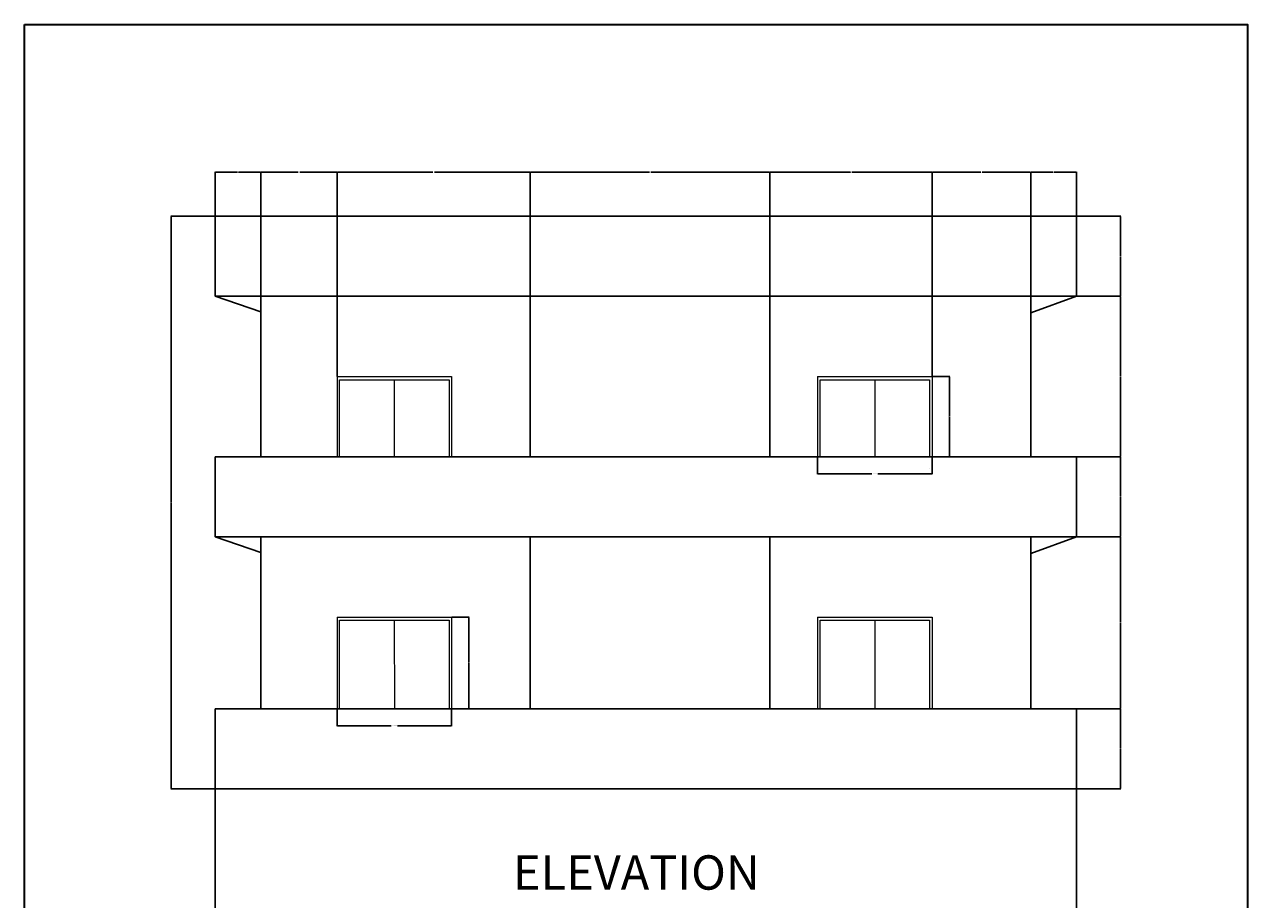
# Model space of a CAD drawing. Units: inches. Extents: x 1854 to 2495, y 1460 to 2772.
# Tile 12 of 12: x 1854 to 2495, y 2314 to 2772. Entities that reach past the tile are written whole.
import ezdxf

# ---------------------------------------------------------------- set-up
doc = ezdxf.new("R2010")
doc.units = ezdxf.units.IN
for name, color, linetype, lineweight in [('A-ANNO-DIMS', 2, 'Continuous', 18), ('A-ANNO-TEXT', 7, 'Continuous', 25), ('A-ANNO-TTLB', 7, 'Continuous', 35), ('A-ELEV', 7, 'Continuous', 25), ('A-ELEV-GLAZ', 4, 'Continuous', 18)]:
    doc.layers.add(name, color=color, linetype=linetype, lineweight=lineweight)
doc.styles.get("Standard").update_dxf_attribs({"font": 'arial.ttf'})
doc.dimstyles.get("Standard").update_dxf_attribs({"dimtxt": 0.18, "dimasz": 0.18, "dimexe": 0.18, "dimexo": 0.0625, "dimgap": 0.09, "dimtad": 0, "dimtih": 1, "dimtoh": 1, "dimdec": 4, "dimzin": 0, "dimdsep": 46, "dimtxsty": 'Standard', "dimcen": 0.09, "dimadec": 0, "dimazin": 0, "dimtfac": 1, "dimtdec": 4, "dimtofl": 0, "dimtmove": 0, "dimatfit": 3, "dimfxl": 1, "dimtolj": 1, "dimtzin": 0, "dimarcsym": 0})

# ---------------------------------------------------------------- blocks, each defined once
blk = doc.blocks.new('ELEV-WINDOW-60X48')
for p, q in [((0, 48), (0, 0)), ((0, 48), (60, 48)), ((29.95, 46.33), (30, 0)), ((60, 48), (60, 0)), ((0, 0), (60, 0))]:
    blk.add_line(p, q)
blk.add_lwpolyline([(1.27, 46.33), (58.63, 46.33), (58.63, 0), (1.27, 0)], close=True)
blk = doc.blocks.new('ELEV-WINDOW-60X42')
for p, q in [((0, 42), (0, 0)), ((0, 42), (60, 42)), ((29.95, 40.33), (29.99, 0)), ((60, 42), (60, 0))]:
    blk.add_line(p, q)
blk.add_lwpolyline([(1.27, 0), (1.27, 40.33), (58.63, 40.33), (58.63, 0)])
blk = doc.blocks.new('*D27')
at = {"layer": 'A-ANNO-DIMS', "color": 0, "lineweight": -2, "transparency": 16777216}
for p, q in [((2017.83, 2414.03), (2017.83, 2404.91)), ((2077.83, 2414.03), (2077.83, 2404.91)), ((2018.01, 2405.09), (2046.22, 2405.09)), ((2077.65, 2405.09), (2049.44, 2405.09))]:
    blk.add_line(p, q, dxfattribs=at)
at = {"layer": 'A-ANNO-DIMS', "color": 0, "transparency": 16777216}
for points in [[(2018.01, 2405.12), (2018.01, 2405.06), (2017.83, 2405.09)], [(2077.65, 2405.12), (2077.65, 2405.06), (2077.83, 2405.09)]]:
    blk.add_solid(points, dxfattribs=at)
at = {"layer": 'Defpoints', "color": 0, "transparency": 16777216}
for p in [(2017.83, 2414.09), (2077.83, 2414.09), (2077.83, 2405.09)]:
    blk.add_point(p, dxfattribs=at)
at = {"layer": 'A-ANNO-DIMS', "color": 0, "transparency": 16777216, "insert": (2047.83, 2405.09), "char_height": 0.18, "attachment_point": 5}
blk.add_mtext('\\A1;LOWER WINDOW 60 TYP.', dxfattribs=at)
blk = doc.blocks.new('*D28')
at = {"layer": 'A-ANNO-DIMS', "color": 0, "lineweight": -2, "transparency": 16777216}
for p, q in [((2077.89, 2462.09), (2087.01, 2462.09)), ((2086.83, 2461.91), (2086.83, 2438.27)), ((2086.83, 2414.27), (2086.83, 2437.91)), ((2077.89, 2414.09), (2087.01, 2414.09))]:
    blk.add_line(p, q, dxfattribs=at)
at = {"layer": 'A-ANNO-DIMS', "color": 0, "transparency": 16777216}
for points in [[(2086.8, 2461.91), (2086.86, 2461.91), (2086.83, 2462.09)], [(2086.8, 2414.27), (2086.86, 2414.27), (2086.83, 2414.09)]]:
    blk.add_solid(points, dxfattribs=at)
at = {"layer": 'Defpoints', "color": 0, "transparency": 16777216}
for p in [(2077.83, 2462.09), (2086.83, 2462.09), (2077.83, 2414.09)]:
    blk.add_point(p, dxfattribs=at)
at = {"layer": 'A-ANNO-DIMS', "color": 0, "transparency": 16777216, "insert": (2086.83, 2438.09), "char_height": 0.18, "attachment_point": 5}
blk.add_mtext('\\A1;48 TYP.', dxfattribs=at)
blk = doc.blocks.new('*D29')
at = {"layer": 'A-ANNO-DIMS', "color": 0, "lineweight": -2, "transparency": 16777216}
for p, q in [((2269.45, 2546.03), (2269.45, 2536.91)), ((2329.45, 2546.03), (2329.45, 2536.91)), ((2269.63, 2537.09), (2297.87, 2537.09)), ((2329.27, 2537.09), (2301.02, 2537.09))]:
    blk.add_line(p, q, dxfattribs=at)
at = {"layer": 'A-ANNO-DIMS', "color": 0, "transparency": 16777216}
for points in [[(2269.63, 2537.12), (2269.63, 2537.06), (2269.45, 2537.09)], [(2329.27, 2537.12), (2329.27, 2537.06), (2329.45, 2537.09)]]:
    blk.add_solid(points, dxfattribs=at)
at = {"layer": 'Defpoints', "color": 0, "transparency": 16777216}
for p in [(2269.45, 2546.09), (2329.45, 2546.09), (2329.45, 2537.09)]:
    blk.add_point(p, dxfattribs=at)
at = {"layer": 'A-ANNO-DIMS', "color": 0, "transparency": 16777216, "insert": (2299.45, 2537.09), "char_height": 0.18, "attachment_point": 5}
blk.add_mtext('\\A1;UPPER WINDOW 60 TYP.', dxfattribs=at)
blk = doc.blocks.new('*D30')
at = {"layer": 'A-ANNO-DIMS', "color": 0, "lineweight": -2, "transparency": 16777216}
for p, q in [((2329.51, 2588.09), (2338.63, 2588.09)), ((2338.45, 2587.91), (2338.45, 2567.27)), ((2338.45, 2546.27), (2338.45, 2566.91)), ((2329.51, 2546.09), (2338.63, 2546.09))]:
    blk.add_line(p, q, dxfattribs=at)
at = {"layer": 'A-ANNO-DIMS', "color": 0, "transparency": 16777216}
for points in [[(2338.42, 2587.91), (2338.48, 2587.91), (2338.45, 2588.09)], [(2338.42, 2546.27), (2338.48, 2546.27), (2338.45, 2546.09)]]:
    blk.add_solid(points, dxfattribs=at)
at = {"layer": 'Defpoints', "color": 0, "transparency": 16777216}
for p in [(2329.45, 2588.09), (2338.45, 2588.09), (2329.45, 2546.09)]:
    blk.add_point(p, dxfattribs=at)
at = {"layer": 'A-ANNO-DIMS', "color": 0, "transparency": 16777216, "insert": (2338.45, 2567.09), "char_height": 0.18, "attachment_point": 5}
blk.add_mtext('\\A1;42 TYP.', dxfattribs=at)
blk = doc.blocks.new('*D74')
at = {"layer": 'A-ANNO-DIMS', "color": 0, "lineweight": -2, "transparency": 16777216}
for p, q in [((1953.98, 2372.03), (1953.98, 2284.46)), ((2404.98, 2372.03), (2404.98, 2284.46)), ((1954.16, 2284.64), (2179.21, 2284.64)), ((2404.8, 2284.64), (2179.76, 2284.64))]:
    blk.add_line(p, q, dxfattribs=at)
at = {"layer": 'A-ANNO-DIMS', "color": 0, "transparency": 16777216}
for points in [[(1954.16, 2284.67), (1954.16, 2284.61), (1953.98, 2284.64)], [(2404.8, 2284.67), (2404.8, 2284.61), (2404.98, 2284.64)]]:
    blk.add_solid(points, dxfattribs=at)
at = {"layer": 'Defpoints', "color": 0, "transparency": 16777216}
for p in [(1953.98, 2372.09), (2404.98, 2372.09), (2404.98, 2284.64)]:
    blk.add_point(p, dxfattribs=at)
at = {"layer": 'A-ANNO-DIMS', "color": 0, "transparency": 16777216, "insert": (2179.48, 2284.64), "char_height": 0.18, "attachment_point": 5}
blk.add_mtext('\\A1;451', dxfattribs=at)
blk = doc.blocks.new('*D75')
at = {"layer": 'A-ANNO-DIMS', "color": 0, "lineweight": -2, "transparency": 16777216}
for p, q in [((1953.92, 2672.09), (1930.75, 2672.09)), ((1930.93, 2671.91), (1930.93, 2522.27)), ((1930.93, 2372.27), (1930.93, 2521.91)), ((1953.92, 2372.09), (1930.75, 2372.09))]:
    blk.add_line(p, q, dxfattribs=at)
at = {"layer": 'A-ANNO-DIMS', "color": 0, "transparency": 16777216}
for points in [[(1930.9, 2671.91), (1930.96, 2671.91), (1930.93, 2672.09)], [(1930.9, 2372.27), (1930.96, 2372.27), (1930.93, 2372.09)]]:
    blk.add_solid(points, dxfattribs=at)
at = {"layer": 'Defpoints', "color": 0, "transparency": 16777216}
for p in [(1930.93, 2672.09), (1953.98, 2672.09), (1953.98, 2372.09)]:
    blk.add_point(p, dxfattribs=at)
at = {"layer": 'A-ANNO-DIMS', "color": 0, "transparency": 16777216, "insert": (1930.93, 2522.09), "char_height": 0.18, "attachment_point": 5}
blk.add_mtext('\\A1;300', dxfattribs=at)
blk = doc.blocks.new('*D76')
at = {"layer": 'A-ANNO-DIMS', "color": 0, "lineweight": -2, "transparency": 16777216}
for p, q in [((2405.04, 2414.09), (2428.21, 2414.09)), ((2428.03, 2413.91), (2428.03, 2393.27)), ((2428.03, 2372.27), (2428.03, 2392.91)), ((2405.04, 2372.09), (2428.21, 2372.09))]:
    blk.add_line(p, q, dxfattribs=at)
at = {"layer": 'A-ANNO-DIMS', "color": 0, "transparency": 16777216}
for points in [[(2428, 2413.91), (2428.06, 2413.91), (2428.03, 2414.09)], [(2428, 2372.27), (2428.06, 2372.27), (2428.03, 2372.09)]]:
    blk.add_solid(points, dxfattribs=at)
at = {"layer": 'Defpoints', "color": 0, "transparency": 16777216}
for p in [(2404.98, 2414.09), (2428.03, 2414.09), (2404.98, 2372.09)]:
    blk.add_point(p, dxfattribs=at)
at = {"layer": 'A-ANNO-DIMS', "color": 0, "transparency": 16777216, "insert": (2428.03, 2393.09), "char_height": 0.18, "attachment_point": 5}
blk.add_mtext('\\A1;42', dxfattribs=at)
blk = doc.blocks.new('*D77')
at = {"layer": 'A-ANNO-DIMS', "color": 0, "lineweight": -2, "transparency": 16777216}
for p, q in [((2405.04, 2504.09), (2428.21, 2504.09)), ((2428.03, 2503.91), (2428.03, 2459.27)), ((2428.03, 2414.27), (2428.03, 2458.91)), ((2405.04, 2414.09), (2428.21, 2414.09))]:
    blk.add_line(p, q, dxfattribs=at)
at = {"layer": 'A-ANNO-DIMS', "color": 0, "transparency": 16777216}
for points in [[(2428, 2503.91), (2428.06, 2503.91), (2428.03, 2504.09)], [(2428, 2414.27), (2428.06, 2414.27), (2428.03, 2414.09)]]:
    blk.add_solid(points, dxfattribs=at)
at = {"layer": 'Defpoints', "color": 0, "transparency": 16777216}
for p in [(2404.98, 2504.09), (2428.03, 2504.09), (2404.98, 2414.09)]:
    blk.add_point(p, dxfattribs=at)
at = {"layer": 'A-ANNO-DIMS', "color": 0, "transparency": 16777216, "insert": (2428.03, 2459.09), "char_height": 0.18, "attachment_point": 5}
blk.add_mtext('\\A1;90', dxfattribs=at)
blk = doc.blocks.new('*D78')
at = {"layer": 'A-ANNO-DIMS', "color": 0, "lineweight": -2, "transparency": 16777216}
for p, q in [((2405.04, 2546.09), (2428.21, 2546.09)), ((2428.03, 2545.91), (2428.03, 2525.27)), ((2428.03, 2504.27), (2428.03, 2524.91)), ((2405.04, 2504.09), (2428.21, 2504.09))]:
    blk.add_line(p, q, dxfattribs=at)
at = {"layer": 'A-ANNO-DIMS', "color": 0, "transparency": 16777216}
for points in [[(2428, 2545.91), (2428.06, 2545.91), (2428.03, 2546.09)], [(2428, 2504.27), (2428.06, 2504.27), (2428.03, 2504.09)]]:
    blk.add_solid(points, dxfattribs=at)
at = {"layer": 'Defpoints', "color": 0, "transparency": 16777216}
for p in [(2404.98, 2546.09), (2428.03, 2546.09), (2404.98, 2504.09)]:
    blk.add_point(p, dxfattribs=at)
at = {"layer": 'A-ANNO-DIMS', "color": 0, "transparency": 16777216, "insert": (2428.03, 2525.09), "char_height": 0.18, "attachment_point": 5}
blk.add_mtext('\\A1;42', dxfattribs=at)
blk = doc.blocks.new('*D79')
at = {"layer": 'A-ANNO-DIMS', "color": 0, "lineweight": -2, "transparency": 16777216}
for p, q in [((2405.04, 2630.09), (2428.21, 2630.09)), ((2428.03, 2629.91), (2428.03, 2588.27)), ((2428.03, 2546.27), (2428.03, 2587.91)), ((2405.04, 2546.09), (2428.21, 2546.09))]:
    blk.add_line(p, q, dxfattribs=at)
at = {"layer": 'A-ANNO-DIMS', "color": 0, "transparency": 16777216}
for points in [[(2428, 2629.91), (2428.06, 2629.91), (2428.03, 2630.09)], [(2428, 2546.27), (2428.06, 2546.27), (2428.03, 2546.09)]]:
    blk.add_solid(points, dxfattribs=at)
at = {"layer": 'Defpoints', "color": 0, "transparency": 16777216}
for p in [(2404.98, 2630.09), (2428.03, 2630.09), (2404.98, 2546.09)]:
    blk.add_point(p, dxfattribs=at)
at = {"layer": 'A-ANNO-DIMS', "color": 0, "transparency": 16777216, "insert": (2428.03, 2588.09), "char_height": 0.18, "attachment_point": 5}
blk.add_mtext('\\A1;84', dxfattribs=at)
blk = doc.blocks.new('*D80')
at = {"layer": 'A-ANNO-DIMS', "color": 0, "lineweight": -2, "transparency": 16777216}
for p, q in [((2405.04, 2672.09), (2428.21, 2672.09)), ((2428.03, 2671.91), (2428.03, 2651.27)), ((2428.03, 2630.27), (2428.03, 2650.91)), ((2405.04, 2630.09), (2428.21, 2630.09))]:
    blk.add_line(p, q, dxfattribs=at)
at = {"layer": 'A-ANNO-DIMS', "color": 0, "transparency": 16777216}
for points in [[(2428, 2671.91), (2428.06, 2671.91), (2428.03, 2672.09)], [(2428, 2630.27), (2428.06, 2630.27), (2428.03, 2630.09)]]:
    blk.add_solid(points, dxfattribs=at)
at = {"layer": 'Defpoints', "color": 0, "transparency": 16777216}
for p in [(2404.98, 2672.09), (2428.03, 2672.09), (2404.98, 2630.09)]:
    blk.add_point(p, dxfattribs=at)
at = {"layer": 'A-ANNO-DIMS', "color": 0, "transparency": 16777216, "insert": (2428.03, 2651.09), "char_height": 0.18, "attachment_point": 5}
blk.add_mtext('\\A1;42', dxfattribs=at)
blk = doc.blocks.new('*D81')
at = {"layer": 'A-ANNO-DIMS', "color": 0, "lineweight": -2, "transparency": 16777216}
for p, q in [((1953.98, 2672.15), (1953.98, 2695.32)), ((1954.16, 2695.14), (1965.76, 2695.14)), ((1977.8, 2695.14), (1966.2, 2695.14)), ((1977.98, 2630.15), (1977.98, 2695.32))]:
    blk.add_line(p, q, dxfattribs=at)
at = {"layer": 'A-ANNO-DIMS', "color": 0, "transparency": 16777216}
for points in [[(1954.16, 2695.17), (1954.16, 2695.11), (1953.98, 2695.14)], [(1977.8, 2695.17), (1977.8, 2695.11), (1977.98, 2695.14)]]:
    blk.add_solid(points, dxfattribs=at)
at = {"layer": 'Defpoints', "color": 0, "transparency": 16777216}
for p in [(1977.98, 2695.14), (1953.98, 2672.09), (1977.98, 2630.09)]:
    blk.add_point(p, dxfattribs=at)
at = {"layer": 'A-ANNO-DIMS', "color": 0, "transparency": 16777216, "insert": (1965.98, 2695.14), "char_height": 0.18, "attachment_point": 5}
blk.add_mtext('\\A1;24', dxfattribs=at)
blk = doc.blocks.new('*D82')
at = {"layer": 'A-ANNO-DIMS', "color": 0, "lineweight": -2, "transparency": 16777216}
for p, q in [((1977.98, 2630.15), (1977.98, 2695.32)), ((1978.16, 2695.14), (1997.51, 2695.14)), ((2017.65, 2695.14), (1998.3, 2695.14)), ((2017.83, 2588.15), (2017.83, 2695.32))]:
    blk.add_line(p, q, dxfattribs=at)
at = {"layer": 'A-ANNO-DIMS', "color": 0, "transparency": 16777216}
for points in [[(1978.16, 2695.17), (1978.16, 2695.11), (1977.98, 2695.14)], [(2017.65, 2695.17), (2017.65, 2695.11), (2017.83, 2695.14)]]:
    blk.add_solid(points, dxfattribs=at)
at = {"layer": 'Defpoints', "color": 0, "transparency": 16777216}
for p in [(2017.83, 2695.14), (1977.98, 2630.09), (2017.83, 2588.09)]:
    blk.add_point(p, dxfattribs=at)
at = {"layer": 'A-ANNO-DIMS', "color": 0, "transparency": 16777216, "insert": (1997.91, 2695.14), "char_height": 0.18, "attachment_point": 5}
blk.add_mtext('\\A1;39.85', dxfattribs=at)
blk = doc.blocks.new('*D83')
at = {"layer": 'A-ANNO-DIMS', "color": 0, "lineweight": -2, "transparency": 16777216}
for p, q in [((2017.83, 2588.15), (2017.83, 2695.32)), ((2018.01, 2695.14), (2067.95, 2695.14)), ((2118.8, 2695.14), (2068.86, 2695.14)), ((2118.98, 2630.15), (2118.98, 2695.32))]:
    blk.add_line(p, q, dxfattribs=at)
at = {"layer": 'A-ANNO-DIMS', "color": 0, "transparency": 16777216}
for points in [[(2018.01, 2695.17), (2018.01, 2695.11), (2017.83, 2695.14)], [(2118.8, 2695.17), (2118.8, 2695.11), (2118.98, 2695.14)]]:
    blk.add_solid(points, dxfattribs=at)
at = {"layer": 'Defpoints', "color": 0, "transparency": 16777216}
for p in [(2118.98, 2695.14), (2118.98, 2630.09), (2017.83, 2588.09)]:
    blk.add_point(p, dxfattribs=at)
at = {"layer": 'A-ANNO-DIMS', "color": 0, "transparency": 16777216, "insert": (2068.41, 2695.14), "char_height": 0.18, "attachment_point": 5}
blk.add_mtext('\\A1;101.15', dxfattribs=at)
blk = doc.blocks.new('*D84')
at = {"layer": 'A-ANNO-DIMS', "color": 0, "lineweight": -2, "transparency": 16777216}
for p, q in [((2118.98, 2630.15), (2118.98, 2695.32)), ((2119.16, 2695.14), (2181.35, 2695.14)), ((2244.3, 2695.14), (2182.12, 2695.14)), ((2244.48, 2630.15), (2244.48, 2695.32))]:
    blk.add_line(p, q, dxfattribs=at)
at = {"layer": 'A-ANNO-DIMS', "color": 0, "transparency": 16777216}
for points in [[(2119.16, 2695.17), (2119.16, 2695.11), (2118.98, 2695.14)], [(2244.3, 2695.17), (2244.3, 2695.11), (2244.48, 2695.14)]]:
    blk.add_solid(points, dxfattribs=at)
at = {"layer": 'Defpoints', "color": 0, "transparency": 16777216}
for p in [(2244.48, 2695.14), (2118.98, 2630.09), (2244.48, 2630.09)]:
    blk.add_point(p, dxfattribs=at)
at = {"layer": 'A-ANNO-DIMS', "color": 0, "transparency": 16777216, "insert": (2181.73, 2695.14), "char_height": 0.18, "attachment_point": 5}
blk.add_mtext('\\A1;125.5', dxfattribs=at)
blk = doc.blocks.new('*D85')
at = {"layer": 'A-ANNO-DIMS', "color": 0, "lineweight": -2, "transparency": 16777216}
for p, q in [((2244.48, 2630.15), (2244.48, 2695.32)), ((2244.66, 2695.14), (2286.57, 2695.14)), ((2329.27, 2695.14), (2287.36, 2695.14)), ((2329.45, 2588.15), (2329.45, 2695.32))]:
    blk.add_line(p, q, dxfattribs=at)
at = {"layer": 'A-ANNO-DIMS', "color": 0, "transparency": 16777216}
for points in [[(2244.66, 2695.17), (2244.66, 2695.11), (2244.48, 2695.14)], [(2329.27, 2695.17), (2329.27, 2695.11), (2329.45, 2695.14)]]:
    blk.add_solid(points, dxfattribs=at)
at = {"layer": 'Defpoints', "color": 0, "transparency": 16777216}
for p in [(2329.45, 2695.14), (2244.48, 2630.09), (2329.45, 2588.09)]:
    blk.add_point(p, dxfattribs=at)
at = {"layer": 'A-ANNO-DIMS', "color": 0, "transparency": 16777216, "insert": (2286.96, 2695.14), "char_height": 0.18, "attachment_point": 5}
blk.add_mtext('\\A1;84.96', dxfattribs=at)
blk = doc.blocks.new('*D86')
at = {"layer": 'A-ANNO-DIMS', "color": 0, "lineweight": -2, "transparency": 16777216}
for p, q in [((2329.45, 2588.15), (2329.45, 2695.32)), ((2329.63, 2695.14), (2354.82, 2695.14)), ((2380.8, 2695.14), (2355.61, 2695.14)), ((2380.98, 2630.15), (2380.98, 2695.32))]:
    blk.add_line(p, q, dxfattribs=at)
at = {"layer": 'A-ANNO-DIMS', "color": 0, "transparency": 16777216}
for points in [[(2329.63, 2695.17), (2329.63, 2695.11), (2329.45, 2695.14)], [(2380.8, 2695.17), (2380.8, 2695.11), (2380.98, 2695.14)]]:
    blk.add_solid(points, dxfattribs=at)
at = {"layer": 'Defpoints', "color": 0, "transparency": 16777216}
for p in [(2380.98, 2695.14), (2380.98, 2630.09), (2329.45, 2588.09)]:
    blk.add_point(p, dxfattribs=at)
at = {"layer": 'A-ANNO-DIMS', "color": 0, "transparency": 16777216, "insert": (2355.21, 2695.14), "char_height": 0.18, "attachment_point": 5}
blk.add_mtext('\\A1;51.54', dxfattribs=at)
blk = doc.blocks.new('*D87')
at = {"layer": 'A-ANNO-DIMS', "color": 0, "lineweight": -2, "transparency": 16777216}
for p, q in [((2380.98, 2630.15), (2380.98, 2695.32)), ((2381.16, 2695.14), (2392.76, 2695.14)), ((2404.8, 2695.14), (2393.2, 2695.14)), ((2404.98, 2672.15), (2404.98, 2695.32))]:
    blk.add_line(p, q, dxfattribs=at)
at = {"layer": 'A-ANNO-DIMS', "color": 0, "transparency": 16777216}
for points in [[(2381.16, 2695.17), (2381.16, 2695.11), (2380.98, 2695.14)], [(2404.8, 2695.17), (2404.8, 2695.11), (2404.98, 2695.14)]]:
    blk.add_solid(points, dxfattribs=at)
at = {"layer": 'Defpoints', "color": 0, "transparency": 16777216}
for p in [(2404.98, 2695.14), (2404.98, 2672.09), (2380.98, 2630.09)]:
    blk.add_point(p, dxfattribs=at)
at = {"layer": 'A-ANNO-DIMS', "color": 0, "transparency": 16777216, "insert": (2392.98, 2695.14), "char_height": 0.18, "attachment_point": 5}
blk.add_mtext('\\A1;24', dxfattribs=at)

msp = doc.modelspace()

# ---------------------------------------------------------------- linework, layer by layer
at = {"layer": 'A-ANNO-TTLB'}
msp.add_lwpolyline([(1854.1764, 2772.4852), (2494.521, 2772.4852), (2494.521, 1460.4076), (1854.1764, 1460.4076)], close=True, dxfattribs=at)
at = {"layer": 'A-ELEV'}
for p, q in [((1953.9824, 2672.0884), (2404.9824, 2672.0884)), ((1953.9824, 2630.0884), (1953.9824, 2672.0884)), ((2404.9824, 2630.0884), (2404.9824, 2672.0884)), ((1953.9824, 2630.0884), (2404.9824, 2630.0884)), ((1953.9824, 2630.0884), (1977.9824, 2621.9559)), ((1977.9824, 2630.0884), (1977.9824, 2546.0884)), ((2118.9824, 2630.0884), (2118.9824, 2546.0884)), ((2244.4824, 2630.0884), (2244.4824, 2546.0884)), ((2244.4824, 2630.0884), (2244.4824, 2546.0884)), ((2380.9824, 2630.0884), (2380.9824, 2546.0884)), ((2404.9824, 2630.0884), (2380.9824, 2621.465)), ((1953.9824, 2546.0884), (2404.9824, 2546.0884)), ((1953.9824, 2504.0884), (1953.9824, 2546.0884)), ((2404.9824, 2504.0884), (2404.9824, 2546.0884)), ((1953.9824, 2504.0884), (2404.9824, 2504.0884)), ((1953.9824, 2504.0884), (1977.9824, 2495.9559)), ((1977.9824, 2504.0884), (1977.9824, 2414.0884)), ((1977.9824, 2504.0884), (1977.9824, 2486.0884)), ((2118.9824, 2504.0884), (2118.9824, 2414.0884)), ((2244.4824, 2504.0884), (2244.4824, 2414.0884)), ((2244.4824, 2504.0884), (2244.4824, 2414.0884)), ((2380.9824, 2504.0884), (2380.9824, 2414.0884)), ((2380.9824, 2504.0884), (2380.9824, 2486.0884)), ((2404.9824, 2504.0884), (2380.9824, 2495.465)), ((1953.9824, 2372.0884), (1953.9824, 2414.0884)), ((1953.9824, 2414.0884), (2404.9824, 2414.0884)), ((2404.9824, 2372.0884), (2404.9824, 2414.0884)), ((1977.9824, 2372.0884), (1953.9824, 2372.0884)), ((1977.9824, 2372.0884), (2380.9824, 2372.0884)), ((2380.9824, 2372.0884), (2380.9824, 2372.0884)), ((2380.9824, 2372.0884), (2404.9824, 2372.0884))]:
    msp.add_line(p, q, dxfattribs=at)
at = {"layer": 'A-ELEV-GLAZ'}
for p, q in [((2017.8299, 2588.0884), (2017.8299, 2546.0884)), ((2017.8299, 2588.0884), (2077.8299, 2588.0884)), ((2077.8299, 2588.0884), (2077.8299, 2546.0884)), ((2269.4451, 2588.0884), (2269.4451, 2546.0884)), ((2269.4451, 2588.0884), (2329.4451, 2588.0884)), ((2329.4451, 2588.0884), (2329.4451, 2546.0884)), ((2329.4451, 2588.0884), (2329.4451, 2546.0884)), ((2269.4451, 2462.0884), (2269.4451, 2414.0884)), ((2269.4451, 2462.0884), (2329.4451, 2462.0884)), ((2329.4451, 2462.0884), (2329.4451, 2414.0884)), ((2329.4451, 2462.0884), (2329.4451, 2414.0884))]:
    msp.add_line(p, q, dxfattribs=at)
msp.add_lwpolyline([(2328.0785, 2540.0884), (2328.0785, 2540.0884)], close=True, dxfattribs=at)

# ---------------------------------------------------------------- block references
for name, p in [('ELEV-WINDOW-60X42', (2017.83, 2546.088)), ('ELEV-WINDOW-60X42', (2269.4452, 2546.088)), ('ELEV-WINDOW-60X48', (2017.83, 2414.088)), ('ELEV-WINDOW-60X48', (2269.4452, 2414.088))]:
    msp.add_blockref(name, p, dxfattribs=at)

# ---------------------------------------------------------------- texts
at = {"layer": 'A-ANNO-TEXT', "insert": (2109.9837, 2337.2946), "char_height": 18, "attachment_point": 1}
msp.add_mtext_dynamic_manual_height_columns('ELEVATION', width=331.684834, gutter_width=12.5, heights=[0], dxfattribs=at)

# ---------------------------------------------------------------- dimensions: what is measured, and where the dimension line sits
at = {"layer": 'A-ANNO-DIMS'}
for base, p1, p2, override, picture, middle in [((1977.9824, 2695.1384), (1953.9824, 2672.0884), (1977.9824, 2630.0884), {"dimdec": 0, "dimlfac": 1, "dimrnd": 0, "dimzin": 0, "dimdsep": 46, "dimlunit": 2}, '*D81', (1965.9824, 2695.1384)), ((2017.8299, 2695.1384), (1977.9824, 2630.0884), (2017.8299, 2588.0884), {"dimdec": 2, "dimlfac": 1, "dimrnd": 0, "dimzin": 0, "dimdsep": 46, "dimlunit": 2}, '*D82', (1997.9061, 2695.1384)), ((2118.9824, 2695.1384), (2017.8299, 2588.0884), (2118.9824, 2630.0884), {"dimdec": 2, "dimlfac": 1, "dimrnd": 0, "dimzin": 0, "dimdsep": 46, "dimlunit": 2}, '*D83', (2068.4061, 2695.1384)), ((2244.4824, 2695.1384), (2118.9824, 2630.0884), (2244.4824, 2630.0884), {"dimdec": 1, "dimlfac": 1, "dimrnd": 0, "dimzin": 0, "dimdsep": 46, "dimlunit": 2}, '*D84', (2181.7324, 2695.1384)), ((2329.4451, 2695.1384), (2244.4824, 2630.0884), (2329.4451, 2588.0884), {"dimdec": 2, "dimlfac": 1, "dimrnd": 0, "dimzin": 0, "dimdsep": 46, "dimlunit": 2}, '*D85', (2286.9638, 2695.1384)), ((2380.9824, 2695.1384), (2329.4451, 2588.0884), (2380.9824, 2630.0884), {"dimdec": 2, "dimlfac": 1, "dimrnd": 0, "dimzin": 0, "dimdsep": 46, "dimlunit": 2}, '*D86', (2355.2138, 2695.1384)), ((2404.9824, 2695.1384), (2380.9824, 2630.0884), (2404.9824, 2672.0884), {"dimdec": 0, "dimlfac": 1, "dimrnd": 0, "dimzin": 0, "dimdsep": 46, "dimlunit": 2}, '*D87', (2392.9824, 2695.1384)), ((2404.9824, 2284.6405), (1953.9824, 2372.0884), (2404.9824, 2372.0884), {"dimdec": 0, "dimlfac": 1, "dimrnd": 0, "dimzin": 0, "dimdsep": 46, "dimlunit": 2}, '*D74', (2179.4824, 2284.6405))]:
    dim = msp.add_linear_dim(base=base, p1=p1, p2=p2, dimstyle='Standard', override=override, dxfattribs=at)
    dim.commit()
    dim.dimension.update_dxf_attribs({"geometry": picture, "text_midpoint": middle})
for base, p1, p2, picture, middle in [((1930.9324, 2672.0884), (1953.9824, 2372.0884), (1953.9824, 2672.0884), '*D75', (1930.9324, 2522.0884)), ((2428.0324, 2672.0884), (2404.9824, 2630.0884), (2404.9824, 2672.0884), '*D80', (2428.0324, 2651.0884)), ((2428.0324, 2630.0884), (2404.9824, 2546.0884), (2404.9824, 2630.0884), '*D79', (2428.0324, 2588.0884)), ((2428.0324, 2546.0884), (2404.9824, 2504.0884), (2404.9824, 2546.0884), '*D78', (2428.0324, 2525.0884)), ((2428.0324, 2504.0884), (2404.9824, 2414.0884), (2404.9824, 2504.0884), '*D77', (2428.0324, 2459.0884)), ((2428.0324, 2414.0884), (2404.9824, 2372.0884), (2404.9824, 2414.0884), '*D76', (2428.0324, 2393.0884))]:
    dim = msp.add_linear_dim(base=base, p1=p1, p2=p2, angle=90, dimstyle='Standard', override={"dimdec": 0, "dimlfac": 1, "dimrnd": 0, "dimzin": 0, "dimdsep": 46, "dimlunit": 2}, dxfattribs=at)
    dim.commit()
    dim.dimension.update_dxf_attribs({"geometry": picture, "text_midpoint": middle})
for base, p1, p2, picture, middle in [((2338.4451, 2588.0884), (2329.4451, 2546.0884), (2329.4451, 2588.0884), '*D30', (2338.4451, 2567.0884)), ((2086.8299, 2462.0884), (2077.8299, 2414.0884), (2077.8299, 2462.0884), '*D28', (2086.8299, 2438.0884))]:
    dim = msp.add_linear_dim(base=base, p1=p1, p2=p2, angle=90, text='<> TYP.', dimstyle='Standard', override={"dimdec": 0, "dimlfac": 1, "dimrnd": 0, "dimzin": 0, "dimdsep": 46, "dimlunit": 2}, dxfattribs=at)
    dim.commit()
    dim.dimension.update_dxf_attribs({"geometry": picture, "text_midpoint": middle})
for base, p1, p2, text, picture, middle in [((2329.4451, 2537.0884), (2269.4451, 2546.0884), (2329.4451, 2546.0884), 'UPPER WINDOW <> TYP.', '*D29', (2299.4451, 2537.0884)), ((2077.8299, 2405.0884), (2017.8299, 2414.0884), (2077.8299, 2414.0884), 'LOWER WINDOW <> TYP.', '*D27', (2047.8299, 2405.0884))]:
    dim = msp.add_linear_dim(base=base, p1=p1, p2=p2, text=text, dimstyle='Standard', override={"dimdec": 0, "dimlfac": 1, "dimrnd": 0, "dimzin": 0, "dimdsep": 46, "dimlunit": 2}, dxfattribs=at)
    dim.commit()
    dim.dimension.update_dxf_attribs({"geometry": picture, "text_midpoint": middle})

doc.saveas('drawing.dxf')
